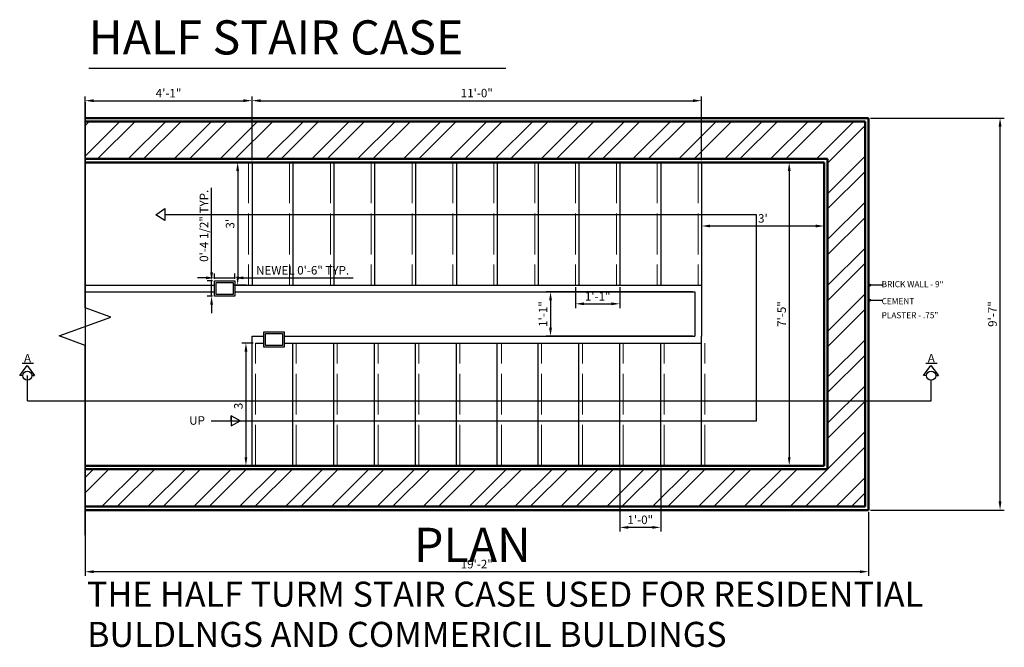
# Model space of a CAD drawing. Units: inches. Extents: x 149 to 438, y 617 to 801.
import ezdxf

# ---------------------------------------------------------------- set-up
doc = ezdxf.new("R2010")
doc.units = ezdxf.units.IN
doc.linetypes.add('ACAD_ISO02W100', pattern=[15, 12, -3])
for name, color, linetype, lineweight in [('A-ANNO-DIMS', 2, 'Continuous', 18), ('A-ANNO-SYMB', 7, 'Continuous', 25), ('A-ANNO-TEXT', 7, 'Continuous', 25), ('A-FLOR-HRAL', 4, 'Continuous', 30), ('A-FLOR-STRS', 7, 'Continuous', 25), ('A-FLOR-STRS-HIDN', 7, 'ACAD_ISO02W100', 18), ('A-WALL', 7, 'Continuous', 50), ('A-WALL-PATT', 8, 'Continuous', 13)]:
    doc.layers.add(name, color=color, linetype=linetype, lineweight=lineweight)
doc.styles.get("Standard").update_dxf_attribs({"font": 'arial.ttf'})
doc.dimstyles.new('ISO-25', dxfattribs={"dimtxt": 2.5, "dimasz": 2.5, "dimexe": 1.25, "dimexo": 0.625, "dimtad": 1, "dimdec": 0, "dimlunit": 3, "dimtxsty": 'Standard', "dimcen": 2.5, "dimadec": 0, "dimazin": 0, "dimtfac": 1, "dimtdec": 0, "dimtmove": 0, "dimatfit": 3, "dimfxl": 1, "dimarcsym": 0})

# ---------------------------------------------------------------- blocks, each defined once
blk = doc.blocks.new('*D2')
at = {"layer": 'A-ANNO-DIMS', "color": 0, "lineweight": -2, "transparency": 16777216}
for p, q in [((215.41, 758.92), (211.57, 758.92)), ((212.82, 756.42), (212.82, 725.42)), ((215.41, 722.92), (211.57, 722.92))]:
    blk.add_line(p, q, dxfattribs=at)
at = {"layer": 'A-ANNO-DIMS', "color": 0, "transparency": 16777216}
for points in [[(212.41, 756.42), (213.24, 756.42), (212.82, 758.92)], [(212.41, 725.42), (213.24, 725.42), (212.82, 722.92)]]:
    blk.add_solid(points, dxfattribs=at)
at = {"layer": 'DEFPOINTS', "color": 0, "transparency": 16777216}
for p in [(216.03, 758.92), (212.82, 722.92), (216.03, 722.92)]:
    blk.add_point(p, dxfattribs=at)
at = {"layer": 'A-ANNO-DIMS', "color": 0, "transparency": 16777216, "insert": (210.92, 740.92), "char_height": 2.5, "attachment_point": 5, "rotation": 90}
blk.add_mtext("3'", dxfattribs=at)
blk = doc.blocks.new('*D3')
at = {"layer": 'A-ANNO-DIMS', "color": 0, "lineweight": -2, "transparency": 16777216}
for p, q in [((384.41, 758.92), (373.5, 758.92)), ((374.75, 756.42), (374.75, 672.42)), ((384.41, 669.92), (373.5, 669.92))]:
    blk.add_line(p, q, dxfattribs=at)
at = {"layer": 'A-ANNO-DIMS', "color": 0, "transparency": 16777216}
for points in [[(374.34, 756.42), (375.17, 756.42), (374.75, 758.92)], [(374.34, 672.42), (375.17, 672.42), (374.75, 669.92)]]:
    blk.add_solid(points, dxfattribs=at)
at = {"layer": 'DEFPOINTS', "color": 0, "transparency": 16777216}
for p in [(385.03, 758.92), (374.75, 669.92), (385.03, 669.92)]:
    blk.add_point(p, dxfattribs=at)
at = {"layer": 'A-ANNO-DIMS', "color": 0, "transparency": 16777216, "insert": (372.86, 714.42), "char_height": 2.5, "attachment_point": 5, "rotation": 90}
blk.add_mtext('7\'-5"', dxfattribs=at)
blk = doc.blocks.new('*D4')
at = {"layer": 'A-ANNO-DIMS', "color": 0, "lineweight": -2, "transparency": 16777216}
for p, q in [((349.03, 758.29), (349.03, 739)), ((385.03, 758.29), (385.03, 739)), ((351.53, 740.25), (382.53, 740.25))]:
    blk.add_line(p, q, dxfattribs=at)
at = {"layer": 'A-ANNO-DIMS', "color": 0, "transparency": 16777216}
for points in [[(351.53, 740.67), (351.53, 739.83), (349.03, 740.25)], [(382.53, 740.67), (382.53, 739.83), (385.03, 740.25)]]:
    blk.add_solid(points, dxfattribs=at)
at = {"layer": 'DEFPOINTS', "color": 0, "transparency": 16777216}
for p in [(349.03, 758.92), (385.03, 758.92), (385.03, 740.25)]:
    blk.add_point(p, dxfattribs=at)
at = {"layer": 'A-ANNO-DIMS', "color": 0, "transparency": 16777216, "insert": (367.03, 742.15), "char_height": 2.5, "attachment_point": 5}
blk.add_mtext("3'", dxfattribs=at)
blk = doc.blocks.new('*D5')
at = {"layer": 'A-ANNO-DIMS', "color": 0, "lineweight": -2, "transparency": 16777216}
for p, q in [((312.03, 722.29), (312.03, 716.17)), ((325.03, 722.29), (325.03, 716.17)), ((314.53, 717.42), (322.53, 717.42))]:
    blk.add_line(p, q, dxfattribs=at)
at = {"layer": 'A-ANNO-DIMS', "color": 0, "transparency": 16777216}
for points in [[(314.53, 717.84), (314.53, 717.01), (312.03, 717.42)], [(322.53, 717.84), (322.53, 717.01), (325.03, 717.42)]]:
    blk.add_solid(points, dxfattribs=at)
at = {"layer": 'DEFPOINTS', "color": 0, "transparency": 16777216}
for p in [(312.03, 722.92), (325.03, 722.92), (325.03, 717.42)]:
    blk.add_point(p, dxfattribs=at)
at = {"layer": 'A-ANNO-DIMS', "color": 0, "transparency": 16777216, "insert": (318.53, 719.3), "char_height": 2.5, "attachment_point": 5}
blk.add_mtext('1\'-1"', dxfattribs=at)
blk = doc.blocks.new('*D6')
at = {"layer": 'A-ANNO-DIMS', "color": 0, "lineweight": -2, "transparency": 16777216}
for p, q in [((346.41, 720.92), (303.43, 720.92)), ((304.68, 718.42), (304.68, 710.42)), ((346.41, 707.92), (303.43, 707.92))]:
    blk.add_line(p, q, dxfattribs=at)
at = {"layer": 'A-ANNO-DIMS', "color": 0, "transparency": 16777216}
for points in [[(304.26, 718.42), (305.1, 718.42), (304.68, 720.92)], [(304.26, 710.42), (305.1, 710.42), (304.68, 707.92)]]:
    blk.add_solid(points, dxfattribs=at)
at = {"layer": 'DEFPOINTS', "color": 0, "transparency": 16777216}
for p in [(347.03, 720.92), (304.68, 707.92), (347.03, 707.92)]:
    blk.add_point(p, dxfattribs=at)
at = {"layer": 'A-ANNO-DIMS', "color": 0, "transparency": 16777216, "insert": (302.8, 714.42), "char_height": 2.5, "attachment_point": 5, "rotation": 90}
blk.add_mtext('1\'-1"', dxfattribs=at)
blk = doc.blocks.new('*D7')
at = {"layer": 'A-ANNO-DIMS', "color": 0, "lineweight": -2, "transparency": 16777216}
for p, q in [((217.41, 705.92), (214, 705.92)), ((215.25, 703.42), (215.25, 672.42)), ((217.41, 669.92), (214, 669.92))]:
    blk.add_line(p, q, dxfattribs=at)
at = {"layer": 'A-ANNO-DIMS', "color": 0, "transparency": 16777216}
for points in [[(214.84, 703.42), (215.67, 703.42), (215.25, 705.92)], [(214.84, 672.42), (215.67, 672.42), (215.25, 669.92)]]:
    blk.add_solid(points, dxfattribs=at)
at = {"layer": 'DEFPOINTS', "color": 0, "transparency": 16777216}
for p in [(218.03, 705.92), (215.25, 669.92), (218.03, 669.92)]:
    blk.add_point(p, dxfattribs=at)
at = {"layer": 'A-ANNO-DIMS', "color": 0, "transparency": 16777216, "insert": (213.35, 687.92), "char_height": 2.5, "attachment_point": 5, "rotation": 90}
blk.add_mtext("3'", dxfattribs=at)
blk = doc.blocks.new('STAIR-NEWEL')
for points in [[(0, 4.46), (5.95, 4.46), (5.95, 0), (0, 0)], [(0.5, 3.96), (5.45, 3.96), (5.45, 0.5), (0.5, 0.5)]]:
    blk.add_lwpolyline(points, close=True)
blk = doc.blocks.new('SECTION-HEAD-A')
for p, q in [((0, 1.36), (2.17, 4.35)), ((0.69, 5.05), (4.04, 5.05)), ((2.17, 4.35), (4.39, 1.36)), ((0.9, 1.36), (0, 1.36)), ((3.61, 1.36), (4.39, 1.36)), ((4.39, 1.36), (3.61, 1.36))]:
    blk.add_line(p, q)
blk.add_circle((2.25, 1.36), 1.36)
at = {"insert": (1.27, 7.75), "char_height": 2.5, "attachment_point": 1}
blk.add_mtext_dynamic_manual_height_columns('A', width=2.2673, gutter_width=12.5, heights=[0], dxfattribs=at)
blk = doc.blocks.new('LEADER-ARROW-OPEN')
for p, q in [((0, 0.28), (0.41, 0.58)), ((0.41, 0), (0, 0.28)), ((0.41, 0.58), (0.41, 0))]:
    blk.add_line(p, q)
blk = doc.blocks.new('*D11')
at = {"layer": 'A-ANNO-DIMS', "color": 0, "lineweight": -2, "transparency": 16777216}
for p, q in [((206.05, 724.76), (206.05, 726.28)), ((212, 724.76), (212, 726.28)), ((203.55, 725.03), (201.05, 725.03)), ((206.05, 725.03), (212, 725.03)), ((214.5, 725.03), (246.76, 725.03))]:
    blk.add_line(p, q, dxfattribs=at)
at = {"layer": 'A-ANNO-DIMS', "color": 0, "transparency": 16777216}
for points in [[(203.55, 725.45), (203.55, 724.62), (206.05, 725.03)], [(214.5, 725.45), (214.5, 724.62), (212, 725.03)]]:
    blk.add_solid(points, dxfattribs=at)
at = {"layer": 'DEFPOINTS', "color": 0, "transparency": 16777216}
for p in [(206.05, 724.14), (212, 725.03), (212, 724.14)]:
    blk.add_point(p, dxfattribs=at)
at = {"layer": 'A-ANNO-DIMS', "color": 0, "transparency": 16777216, "insert": (231.88, 726.93), "char_height": 2.5, "attachment_point": 5}
blk.add_mtext('NEWEL 0\'-6" TYP.', dxfattribs=at)
blk = doc.blocks.new('*D12')
at = {"layer": 'A-ANNO-DIMS', "color": 0, "lineweight": -2, "transparency": 16777216}
for p, q in [((205.16, 726.64), (205.16, 751.45)), ((205.43, 724.14), (203.91, 724.14)), ((205.16, 719.68), (205.16, 724.14)), ((205.43, 719.68), (203.91, 719.68)), ((205.16, 717.18), (205.16, 714.68))]:
    blk.add_line(p, q, dxfattribs=at)
at = {"layer": 'A-ANNO-DIMS', "color": 0, "transparency": 16777216}
for points in [[(204.74, 726.64), (205.58, 726.64), (205.16, 724.14)], [(204.74, 717.18), (205.58, 717.18), (205.16, 719.68)]]:
    blk.add_solid(points, dxfattribs=at)
at = {"layer": 'DEFPOINTS', "color": 0, "transparency": 16777216}
for p in [(205.16, 724.14), (206.05, 724.14), (206.05, 719.68)]:
    blk.add_point(p, dxfattribs=at)
at = {"layer": 'A-ANNO-DIMS', "color": 0, "transparency": 16777216, "insert": (203.24, 740.3), "char_height": 2.5, "attachment_point": 5, "rotation": 90}
blk.add_mtext('0\'-4 1/2" TYP.', dxfattribs=at)
blk = doc.blocks.new('*D13')
at = {"layer": 'A-ANNO-DIMS', "color": 0, "lineweight": -2, "transparency": 16777216}
for p, q in [((168.02, 656.29), (168.02, 637.57)), ((398.03, 656.29), (398.03, 637.57)), ((395.53, 638.82), (170.52, 638.82))]:
    blk.add_line(p, q, dxfattribs=at)
at = {"layer": 'A-ANNO-DIMS', "color": 0, "transparency": 16777216}
for points in [[(170.52, 639.23), (170.52, 638.4), (168.02, 638.82)], [(395.53, 639.23), (395.53, 638.4), (398.03, 638.82)]]:
    blk.add_solid(points, dxfattribs=at)
at = {"layer": 'DEFPOINTS', "color": 0, "transparency": 16777216}
for p in [(168.02, 656.92), (398.03, 656.92), (168.02, 638.82)]:
    blk.add_point(p, dxfattribs=at)
at = {"layer": 'A-ANNO-DIMS', "color": 0, "transparency": 16777216, "insert": (283.02, 640.72), "char_height": 2.5, "attachment_point": 5}
blk.add_mtext('19\'-2"', dxfattribs=at)
blk = doc.blocks.new('*D14')
at = {"layer": 'A-ANNO-DIMS', "color": 0, "lineweight": -2, "transparency": 16777216}
for p, q in [((398.66, 771.92), (437.91, 771.92)), ((436.66, 659.42), (436.66, 769.42)), ((398.66, 656.92), (437.91, 656.92))]:
    blk.add_line(p, q, dxfattribs=at)
at = {"layer": 'A-ANNO-DIMS', "color": 0, "transparency": 16777216}
for points in [[(436.24, 769.42), (437.07, 769.42), (436.66, 771.92)], [(436.24, 659.42), (437.07, 659.42), (436.66, 656.92)]]:
    blk.add_solid(points, dxfattribs=at)
at = {"layer": 'DEFPOINTS', "color": 0, "transparency": 16777216}
for p in [(398.03, 771.92), (436.66, 771.92), (398.03, 656.92)]:
    blk.add_point(p, dxfattribs=at)
at = {"layer": 'A-ANNO-DIMS', "color": 0, "transparency": 16777216, "insert": (434.76, 714.42), "char_height": 2.5, "attachment_point": 5, "rotation": 90}
blk.add_mtext('9\'-7"', dxfattribs=at)
blk = doc.blocks.new('*D15')
at = {"layer": 'A-ANNO-DIMS', "color": 0, "lineweight": -2, "transparency": 16777216}
for p, q in [((217.03, 759.54), (217.03, 778.27)), ((349.03, 759.54), (349.03, 778.27)), ((219.53, 777.02), (346.53, 777.02))]:
    blk.add_line(p, q, dxfattribs=at)
at = {"layer": 'A-ANNO-DIMS', "color": 0, "transparency": 16777216}
for points in [[(219.53, 777.43), (219.53, 776.6), (217.03, 777.02)], [(346.53, 777.43), (346.53, 776.6), (349.03, 777.02)]]:
    blk.add_solid(points, dxfattribs=at)
at = {"layer": 'DEFPOINTS', "color": 0, "transparency": 16777216}
for p in [(349.03, 777.02), (217.03, 758.92), (349.03, 758.92)]:
    blk.add_point(p, dxfattribs=at)
at = {"layer": 'A-ANNO-DIMS', "color": 0, "transparency": 16777216, "insert": (283.03, 778.92), "char_height": 2.5, "attachment_point": 5}
blk.add_mtext('11\'-0"', dxfattribs=at)
blk = doc.blocks.new('*D16')
at = {"layer": 'A-ANNO-DIMS', "color": 0, "lineweight": -2, "transparency": 16777216}
for p, q in [((168.02, 759.54), (168.02, 778.27)), ((217.03, 759.54), (217.03, 778.27)), ((170.52, 777.02), (214.53, 777.02))]:
    blk.add_line(p, q, dxfattribs=at)
at = {"layer": 'A-ANNO-DIMS', "color": 0, "transparency": 16777216}
for points in [[(170.52, 777.43), (170.52, 776.6), (168.02, 777.02)], [(214.53, 777.43), (214.53, 776.6), (217.03, 777.02)]]:
    blk.add_solid(points, dxfattribs=at)
at = {"layer": 'DEFPOINTS', "color": 0, "transparency": 16777216}
for p in [(217.03, 777.02), (168.02, 758.92), (217.03, 758.92)]:
    blk.add_point(p, dxfattribs=at)
at = {"layer": 'A-ANNO-DIMS', "color": 0, "transparency": 16777216, "insert": (192.52, 778.9), "char_height": 2.5, "attachment_point": 5}
blk.add_mtext('4\'-1"', dxfattribs=at)
blk = doc.blocks.new('*D17')
at = {"layer": 'A-ANNO-DIMS', "color": 0, "lineweight": -2, "transparency": 16777216}
for p, q in [((325.03, 669.29), (325.03, 650.57)), ((337.03, 669.29), (337.03, 650.57)), ((334.53, 651.82), (327.53, 651.82))]:
    blk.add_line(p, q, dxfattribs=at)
at = {"layer": 'A-ANNO-DIMS', "color": 0, "transparency": 16777216}
for points in [[(327.53, 652.23), (327.53, 651.4), (325.03, 651.82)], [(334.53, 652.23), (334.53, 651.4), (337.03, 651.82)]]:
    blk.add_solid(points, dxfattribs=at)
at = {"layer": 'DEFPOINTS', "color": 0, "transparency": 16777216}
for p in [(325.03, 669.92), (337.03, 669.92), (325.03, 651.82)]:
    blk.add_point(p, dxfattribs=at)
at = {"layer": 'A-ANNO-DIMS', "color": 0, "transparency": 16777216, "insert": (331.03, 653.72), "char_height": 2.5, "attachment_point": 5}
blk.add_mtext('1\'-0"', dxfattribs=at)

msp = doc.modelspace()

# ---------------------------------------------------------------- hatches: boundary and pattern name
at = {"layer": 'A-WALL-PATT'}
h = msp.add_hatch(dxfattribs=at)
h.set_pattern_fill('ANSI32', color=256)
h.paths.add_polyline_path([(397.03, 688.99), (386.03, 688.99), (386.03, 668.92), (168.02, 668.92), (168.02, 657.92), (397.03, 657.92)])
h.paths.add_polyline_path([(397.03, 770.92), (386.03, 770.92), (168.02, 770.92), (168.02, 759.92), (386.03, 759.92), (386.03, 688.99), (397.03, 688.99)])

# ---------------------------------------------------------------- linework, layer by layer
at = {"layer": 'A-ANNO-SYMB'}
for p, q in [((168.02, 776.62), (168.02, 649.72)), ((188.84, 743.55), (191.4, 745.41)), ((191.4, 741.84), (188.84, 743.55)), ((191.4, 745.41), (191.4, 741.84)), ((365.13, 743.55), (191.4, 743.55)), ((365.13, 683.04), (365.13, 743.55)), ((151.08, 688.99), (151.08, 696.34)), ((416.42, 688.99), (416.42, 694.99)), ((151.08, 688.99), (416.42, 688.99)), ((205.02, 683.04), (365.13, 683.04)), ((210.87, 683.04), (210.87, 684.52)), ((210.87, 684.52), (210.87, 681.63)), ((213.57, 683.04), (210.87, 684.52)), ((210.87, 681.63), (213.57, 683.04))]:
    msp.add_line(p, q, dxfattribs=at)
msp.add_lwpolyline([(168.02, 649.56), (168.02, 705.22), (160.43, 707.98), (175.6, 713.5), (168.02, 716.26), (168.02, 764.56)], dxfattribs=at)
at = {"layer": 'A-ANNO-TEXT'}
for p, q in [((169.16, 786.57), (291.55, 786.57)), ((402.08, 722.88), (398.5, 722.88)), ((402.13, 718.44), (398.5, 718.44))]:
    msp.add_line(p, q, dxfattribs=at)
at = {"layer": 'A-FLOR-HRAL'}
for p, q in [((168.02, 722.92), (206.05, 722.92)), ((212, 722.92), (349.03, 722.92)), ((168.02, 720.92), (206.05, 720.92)), ((212, 720.92), (347.03, 720.92)), ((347.03, 720.92), (347.03, 707.92)), ((349.03, 720.92), (349.03, 707.92)), ((217.03, 707.92), (220.54, 707.92)), ((218.03, 705.92), (220.54, 705.92)), ((226.49, 707.92), (347.03, 707.92)), ((226.49, 705.92), (349.03, 705.92))]:
    msp.add_line(p, q, dxfattribs=at)
at = {"layer": 'A-FLOR-STRS'}
for p, q in [((217.03, 758.92), (217.03, 722.92)), ((229.03, 758.92), (229.03, 722.92)), ((241.03, 758.92), (241.03, 722.92)), ((253.03, 758.92), (253.03, 722.92)), ((265.03, 758.92), (265.03, 722.92)), ((277.03, 758.92), (277.03, 722.92)), ((289.03, 758.92), (289.03, 722.92)), ((301.03, 758.92), (301.03, 722.92)), ((313.03, 758.92), (313.03, 722.92)), ((325.03, 758.92), (325.03, 722.92)), ((337.03, 758.92), (337.03, 722.92)), ((349.03, 758.92), (349.03, 720.92)), ((217.03, 669.92), (217.03, 707.92)), ((229.03, 669.92), (229.03, 705.92)), ((241.03, 669.92), (241.03, 705.92)), ((253.03, 669.92), (253.03, 705.92)), ((265.03, 669.92), (265.03, 705.92)), ((277.03, 669.92), (277.03, 705.92)), ((289.03, 669.92), (289.03, 705.92)), ((301.03, 669.92), (301.03, 705.92)), ((313.03, 669.92), (313.03, 705.92)), ((325.03, 669.92), (325.03, 705.92)), ((337.03, 669.92), (337.03, 705.92)), ((349.03, 669.92), (349.03, 707.92))]:
    msp.add_line(p, q, dxfattribs=at)
at = {"layer": 'A-FLOR-STRS-HIDN'}
for p, q in [((216.03, 758.92), (216.03, 722.92)), ((228.03, 758.92), (228.03, 722.92)), ((240.03, 758.92), (240.03, 722.92)), ((252.03, 758.92), (252.03, 722.92)), ((264.03, 758.92), (264.03, 722.92)), ((276.03, 758.92), (276.03, 722.92)), ((288.03, 758.92), (288.03, 722.92)), ((300.03, 758.92), (300.03, 722.92)), ((312.03, 758.92), (312.03, 722.92)), ((324.03, 758.92), (324.03, 722.92)), ((336.03, 758.92), (336.03, 722.92)), ((348.03, 758.92), (348.03, 722.92)), ((218.03, 669.92), (218.03, 705.92)), ((230.03, 669.92), (230.03, 705.92)), ((242.03, 669.92), (242.03, 705.92)), ((254.03, 669.92), (254.03, 705.92)), ((266.03, 669.92), (266.03, 705.92)), ((278.03, 669.92), (278.03, 705.92)), ((290.3, 669.92), (290.3, 705.92)), ((302.03, 669.92), (302.03, 705.92)), ((314.03, 669.92), (314.03, 705.92)), ((326.03, 669.92), (326.03, 705.92)), ((338.03, 669.92), (338.03, 705.92)), ((350.03, 669.92), (350.03, 705.92))]:
    msp.add_line(p, q, dxfattribs=at)
at = {"layer": 'A-WALL'}
for p, q in [((168.02, 771.92), (386.03, 771.92)), ((386.03, 771.92), (398.03, 771.92)), ((398.03, 771.92), (398.03, 656.92)), ((168.02, 770.92), (397.03, 770.92)), ((386.03, 770.92), (397.03, 770.92)), ((397.03, 770.92), (397.03, 657.92)), ((168.02, 759.92), (386.03, 759.92)), ((168.02, 758.92), (385.03, 758.92)), ((385.03, 758.92), (385.03, 669.92)), ((385.03, 758.92), (385.03, 705.92)), ((386.03, 759.92), (386.03, 668.92)), ((385.03, 669.92), (168.02, 669.92)), ((386.03, 668.92), (168.02, 668.92)), ((397.03, 657.92), (168.02, 657.92)), ((385.03, 656.92), (168.02, 656.92)), ((385.03, 656.92), (398.03, 656.92))]:
    msp.add_line(p, q, dxfattribs=at)

# ---------------------------------------------------------------- block references
at = {"layer": 'A-ANNO-SYMB'}
for p in [(148.82, 694.98), (414.17, 694.98)]:
    msp.add_blockref('SECTION-HEAD-A', p, dxfattribs=at)
at = {"layer": 'A-ANNO-TEXT'}
for p in [(398.09, 722.6), (398.09, 718.16)]:
    msp.add_blockref('LEADER-ARROW-OPEN', p, dxfattribs=at)
at = {"layer": 'A-FLOR-HRAL'}
for p in [(206.05, 719.68), (220.54, 704.73)]:
    msp.add_blockref('STAIR-NEWEL', p, dxfattribs=at)

# ---------------------------------------------------------------- texts
at = {"layer": 'A-ANNO-TEXT'}
for s, height, p in [('HALF STAIR CASE ', 10.0256, (169.11, 790.57)), ('BRICK WALL - 9"', 1.778, (401.89, 722.29)), ('CEMENT', 1.778, (401.89, 717.31)), ('PLASTER - .75"', 1.778, (401.89, 713.18)), ('PLAN', 10.026, (264.59, 641.69)), ('THE HALF TURM STAIR CASE USED FOR RESIDENTIAL ', 7.3373, (168.61, 628.56)), ('BULDLNGS AND COMMERICIL BULDINGS ', 7.3373, (168.61, 616.77))]:
    msp.add_text(s, height=height, dxfattribs=at).set_placement(p)
at = {"layer": 'A-ANNO-TEXT', "insert": (198.59, 684.44), "char_height": 2.5, "attachment_point": 1}
msp.add_mtext_dynamic_manual_height_columns('UP', width=2.2673, gutter_width=12.5, heights=[0], dxfattribs=at)

# ---------------------------------------------------------------- dimensions: what is measured, and where the dimension line sits
at = {"layer": 'A-ANNO-DIMS'}
for base, p1, p2, override, picture, middle in [((217.03, 777.02), (168.02, 758.92), (217.03, 758.92), {"dimdec": 1, "dimlfac": 1, "dimrnd": 0, "dimzin": 1, "dimdsep": 46, "dimlunit": 4, "dimfrac": 2}, '*D16', (192.52, 778.9)), ((349.03, 777.02), (217.03, 758.92), (349.03, 758.92), {"dimdec": 1, "dimlfac": 1, "dimrnd": 0, "dimzin": 1, "dimdsep": 46, "dimlunit": 4, "dimfrac": 2}, '*D15', (283.03, 778.92)), ((385.03, 740.25), (349.03, 758.92), (385.03, 758.92), {"dimclrd": 0, "dimclre": 0, "dimclrt": 0}, '*D4', (367.03, 742.15)), ((325.03, 717.42), (312.03, 722.92), (325.03, 722.92), {"dimclrd": 0, "dimclre": 0, "dimclrt": 0}, '*D5', (318.53, 719.3))]:
    dim = msp.add_linear_dim(base=base, p1=p1, p2=p2, dimstyle='ISO-25', override=override, dxfattribs=at)
    dim.commit()
    dim.dimension.update_dxf_attribs({"geometry": picture, "text_midpoint": middle})
for base, p1, p2, angle, override, picture, middle in [((436.66, 771.92), (398.03, 656.92), (398.03, 771.92), 90, {"dimdec": 1, "dimlfac": 1, "dimrnd": 0, "dimzin": 1, "dimdsep": 46, "dimlunit": 4, "dimfrac": 2}, '*D14', (434.76, 714.42)), ((212.82, 722.92), (216.03, 758.92), (216.03, 722.92), 90, {"dimclrd": 0, "dimclre": 0, "dimclrt": 0}, '*D2', (210.92, 740.92)), ((374.75, 669.92), (385.03, 758.92), (385.03, 669.92), 90, {"dimclrd": 0, "dimclre": 0, "dimclrt": 0}, '*D3', (372.86, 714.42)), ((304.68, 707.92), (347.03, 720.92), (347.03, 707.92), 90, {"dimclrd": 0, "dimclre": 0, "dimclrt": 0}, '*D6', (302.8, 714.42)), ((215.25, 669.92), (218.03, 705.92), (218.03, 669.92), 90, {"dimclrd": 0, "dimclre": 0, "dimclrt": 0}, '*D7', (213.35, 687.92)), ((325.03, 651.82), (337.03, 669.92), (325.03, 669.92), 180, {"dimdec": 1, "dimlfac": 1, "dimrnd": 0, "dimzin": 1, "dimdsep": 46, "dimlunit": 4, "dimfrac": 2}, '*D17', (331.03, 653.72)), ((168.02, 638.82), (398.03, 656.92), (168.02, 656.92), 180, {"dimdec": 1, "dimlfac": 1, "dimrnd": 0, "dimzin": 1, "dimdsep": 46, "dimlunit": 4, "dimfrac": 2}, '*D13', (283.02, 640.72))]:
    dim = msp.add_linear_dim(base=base, p1=p1, p2=p2, angle=angle, dimstyle='ISO-25', override=override, dxfattribs=at)
    dim.commit()
    dim.dimension.update_dxf_attribs({"geometry": picture, "text_midpoint": middle})
dim = msp.add_linear_dim(base=(205.16, 724.14), p1=(206.05, 719.68), p2=(206.05, 724.14), angle=90, text='<> TYP.', dimstyle='ISO-25', override={"dimdec": 1, "dimlfac": 1, "dimrnd": 0, "dimzin": 1, "dimdsep": 46, "dimlunit": 4, "dimfrac": 2}, dxfattribs=at)
dim.commit()
dim.dimension.update_dxf_attribs({"geometry": '*D12', "text_midpoint": (203.24, 740.3)})
dim = msp.add_linear_dim(base=(212.0018, 725.0324), p1=(206.0523, 724.14), p2=(212.0018, 724.14), text='NEWEL <> TYP.', dimstyle='ISO-25', override={"dimdec": 1, "dimlfac": 1, "dimrnd": 0, "dimzin": 1, "dimdsep": 46, "dimlunit": 4, "dimfrac": 2}, dxfattribs=at)
dim.commit()
dim.dimension.update_dxf_attribs({"geometry": '*D11', "text_midpoint": (231.8808, 726.9339)})

doc.saveas('drawing.dxf')
